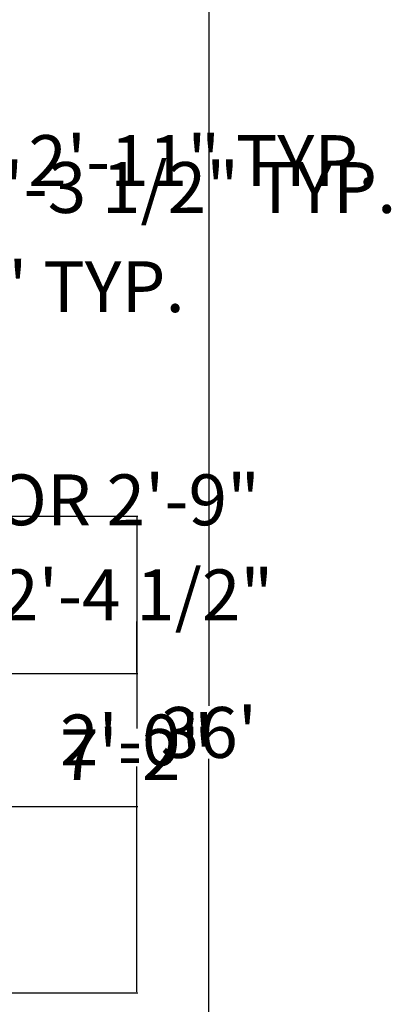
# Model space of a CAD drawing. Units: inches. Extents: x 1086 to 1540, y 3343 to 3848.
# Tile 7 of 8: x 1473 to 1540, y 3547 to 3724. Entities that reach past the tile are written whole.
import ezdxf

# ---------------------------------------------------------------- set-up
doc = ezdxf.new("R2010")
doc.units = ezdxf.units.IN
doc.layers.add('A-ANNO-DIMS', color=2, linetype='Continuous', lineweight=13)
doc.styles.get("Standard").update_dxf_attribs({"font": 'arial.ttf'})
doc.dimstyles.get("Standard").update_dxf_attribs({"dimtxt": 9.18, "dimasz": 0.18, "dimexe": 0.18, "dimexo": 0.0625, "dimgap": 0.09, "dimtad": 0, "dimtih": 1, "dimtoh": 1, "dimdec": 1, "dimzin": 0, "dimdsep": 46, "dimlunit": 3, "dimtxsty": 'Standard', "dimcen": 0.09, "dimadec": 0, "dimazin": 0, "dimtfac": 1, "dimtdec": 1, "dimtofl": 0, "dimtmove": 0, "dimatfit": 3, "dimfxl": 1, "dimtolj": 1, "dimtzin": 0, "dimarcsym": 0})

# ---------------------------------------------------------------- blocks, each defined once
blk = doc.blocks.new('*D13')
at = {"layer": 'A-ANNO-DIMS', "color": 0, "lineweight": -2, "transparency": 16777216}
for p, q in [((1470.8, 3811.57), (1506.93, 3811.57)), ((1506.75, 3811.39), (1506.75, 3600.35)), ((1506.75, 3379.75), (1506.75, 3590.79)), ((1470.8, 3379.57), (1506.93, 3379.57))]:
    blk.add_line(p, q, dxfattribs=at)
at = {"layer": 'A-ANNO-DIMS', "color": 0, "transparency": 16777216}
for points in [[(1506.72, 3811.39), (1506.78, 3811.39), (1506.75, 3811.57)], [(1506.72, 3379.75), (1506.78, 3379.75), (1506.75, 3379.57)]]:
    blk.add_solid(points, dxfattribs=at)
at = {"layer": 'Defpoints', "color": 0, "transparency": 16777216}
for p in [(1470.74, 3811.57), (1470.74, 3379.57), (1506.75, 3379.57)]:
    blk.add_point(p, dxfattribs=at)
at = {"layer": 'A-ANNO-DIMS', "color": 0, "transparency": 16777216, "insert": (1506.75, 3595.57), "char_height": 9.18, "attachment_point": 5}
blk.add_mtext("\\A1;36'", dxfattribs=at)
blk = doc.blocks.new('*D27')
at = {"layer": 'A-ANNO-DIMS', "color": 0, "lineweight": -2, "transparency": 16777216}
for p, q in [((1408.96, 3695.2), (1404.91, 3698.73)), ((1405.05, 3698.61), (1405.16, 3698.75)), ((1405.16, 3698.75), (1405.34, 3698.75)), ((1382.16, 3672.32), (1404.93, 3698.48)), ((1385.96, 3668.77), (1381.9, 3672.3))]:
    blk.add_line(p, q, dxfattribs=at)
at = {"layer": 'A-ANNO-DIMS', "color": 0, "transparency": 16777216}
for points in [[(1404.9, 3698.5), (1404.95, 3698.46), (1405.05, 3698.61)], [(1382.14, 3672.34), (1382.18, 3672.3), (1382.04, 3672.18)]]:
    blk.add_solid(points, dxfattribs=at)
at = {"layer": 'Defpoints', "color": 0, "transparency": 16777216}
for p in [(1405.05, 3698.61), (1409.01, 3695.16), (1386, 3668.73)]:
    blk.add_point(p, dxfattribs=at)
at = {"layer": 'A-ANNO-DIMS', "color": 0, "transparency": 16777216, "insert": (1473.23, 3698.75), "char_height": 9.18, "attachment_point": 5}
blk.add_mtext('\\A1;ARMCHAIR 2\'-11" TYP.', dxfattribs=at)
blk = doc.blocks.new('*D28')
at = {"layer": 'A-ANNO-DIMS', "color": 0, "lineweight": -2, "transparency": 16777216}
for p, q in [((1409.05, 3695.21), (1412.58, 3699.26)), ((1412.6, 3699.01), (1438.75, 3676.24)), ((1435.48, 3672.2), (1439.01, 3676.26)), ((1438.89, 3676.12), (1439.02, 3676)), ((1439.02, 3676), (1439.2, 3676))]:
    blk.add_line(p, q, dxfattribs=at)
at = {"layer": 'A-ANNO-DIMS', "color": 0, "transparency": 16777216}
for points in [[(1412.62, 3699.03), (1412.58, 3698.98), (1412.46, 3699.13)], [(1438.77, 3676.26), (1438.73, 3676.22), (1438.89, 3676.12)]]:
    blk.add_solid(points, dxfattribs=at)
at = {"layer": 'Defpoints', "color": 0, "transparency": 16777216}
for p in [(1409.01, 3695.16), (1438.89, 3676.12), (1435.44, 3672.16)]:
    blk.add_point(p, dxfattribs=at)
at = {"layer": 'A-ANNO-DIMS', "color": 0, "transparency": 16777216, "insert": (1470.92, 3676), "char_height": 9.18, "attachment_point": 5}
blk.add_mtext('\\A1;2\'-11" TYP.', dxfattribs=at)
blk = doc.blocks.new('*D31')
at = {"layer": 'A-ANNO-DIMS', "color": 0, "lineweight": -2, "transparency": 16777216}
for p, q in [((1461.8, 3713.61), (1467.84, 3713.61)), ((1467.66, 3713.43), (1467.66, 3698.73)), ((1467.66, 3674.34), (1467.66, 3689.04)), ((1461.8, 3674.16), (1467.84, 3674.16))]:
    blk.add_line(p, q, dxfattribs=at)
at = {"layer": 'A-ANNO-DIMS', "color": 0, "transparency": 16777216}
for points in [[(1467.63, 3713.43), (1467.69, 3713.43), (1467.66, 3713.61)], [(1467.63, 3674.34), (1467.69, 3674.34), (1467.66, 3674.16)]]:
    blk.add_solid(points, dxfattribs=at)
at = {"layer": 'Defpoints', "color": 0, "transparency": 16777216}
for p in [(1461.74, 3713.61), (1461.74, 3674.16), (1467.66, 3674.16)]:
    blk.add_point(p, dxfattribs=at)
at = {"layer": 'A-ANNO-DIMS', "color": 0, "transparency": 16777216, "insert": (1467.66, 3693.89), "char_height": 9.18, "attachment_point": 5}
blk.add_mtext('\\A1;BOOKCASE 3\'-3 1/2" TYP.', dxfattribs=at)
blk = doc.blocks.new('*D41')
at = {"layer": 'A-ANNO-DIMS', "color": 0, "lineweight": -2, "transparency": 16777216}
for p, q in [((1369.71, 3632.63), (1369.71, 3637.72)), ((1369.89, 3637.54), (1402.67, 3637.54)), ((1402.85, 3632.63), (1402.85, 3637.72)), ((1402.85, 3637.54), (1403.03, 3637.54))]:
    blk.add_line(p, q, dxfattribs=at)
at = {"layer": 'A-ANNO-DIMS', "color": 0, "transparency": 16777216}
for points in [[(1369.89, 3637.57), (1369.89, 3637.51), (1369.71, 3637.54)], [(1402.67, 3637.57), (1402.67, 3637.51), (1402.85, 3637.54)]]:
    blk.add_solid(points, dxfattribs=at)
at = {"layer": 'Defpoints', "color": 0, "transparency": 16777216}
for p in [(1402.85, 3637.54), (1369.71, 3632.57), (1402.85, 3632.57)]:
    blk.add_point(p, dxfattribs=at)
at = {"layer": 'A-ANNO-DIMS', "color": 0, "transparency": 16777216, "insert": (1460.68, 3637.54), "char_height": 9.18, "attachment_point": 5}
blk.add_mtext('\\A1;TOILET DOOR 2\'-9"', dxfattribs=at)
blk = doc.blocks.new('*D67')
at = {"layer": 'A-ANNO-DIMS', "color": 0, "lineweight": -2, "transparency": 16777216}
for p, q in [((1425.8, 3606.21), (1493.92, 3606.21)), ((1493.74, 3606.03), (1493.74, 3598.99)), ((1493.74, 3582.39), (1493.74, 3589.44)), ((1425.8, 3582.21), (1493.92, 3582.21))]:
    blk.add_line(p, q, dxfattribs=at)
at = {"layer": 'A-ANNO-DIMS', "color": 0, "transparency": 16777216}
for points in [[(1493.71, 3606.03), (1493.77, 3606.03), (1493.74, 3606.21)], [(1493.71, 3582.39), (1493.77, 3582.39), (1493.74, 3582.21)]]:
    blk.add_solid(points, dxfattribs=at)
at = {"layer": 'Defpoints', "color": 0, "transparency": 16777216}
for p in [(1425.74, 3606.21), (1493.74, 3606.21), (1425.74, 3582.21)]:
    blk.add_point(p, dxfattribs=at)
at = {"layer": 'A-ANNO-DIMS', "color": 0, "transparency": 16777216, "insert": (1493.74, 3594.21), "char_height": 9.18, "attachment_point": 5}
blk.add_mtext('\\A1;2\'-0"', dxfattribs=at)
blk = doc.blocks.new('*D68')
at = {"layer": 'A-ANNO-DIMS', "color": 0, "lineweight": -2, "transparency": 16777216}
for p, q in [((1425.8, 3634.57), (1493.92, 3634.57)), ((1493.74, 3634.39), (1493.74, 3625.23)), ((1493.74, 3606.39), (1493.74, 3615.56)), ((1425.8, 3606.21), (1493.92, 3606.21))]:
    blk.add_line(p, q, dxfattribs=at)
at = {"layer": 'A-ANNO-DIMS', "color": 0, "transparency": 16777216}
for points in [[(1493.71, 3634.39), (1493.77, 3634.39), (1493.74, 3634.57)], [(1493.71, 3606.39), (1493.77, 3606.39), (1493.74, 3606.21)]]:
    blk.add_solid(points, dxfattribs=at)
at = {"layer": 'Defpoints', "color": 0, "transparency": 16777216}
for p in [(1425.74, 3634.57), (1493.74, 3634.57), (1425.74, 3606.21)]:
    blk.add_point(p, dxfattribs=at)
at = {"layer": 'A-ANNO-DIMS', "color": 0, "transparency": 16777216, "insert": (1493.74, 3620.39), "char_height": 9.18, "attachment_point": 5}
blk.add_mtext('\\A1;2\'-4 1/2"', dxfattribs=at)
blk = doc.blocks.new('*D71')
at = {"layer": 'A-ANNO-DIMS', "color": 0, "lineweight": -2, "transparency": 16777216}
for p, q in [((1461.8, 3634.57), (1493.92, 3634.57)), ((1493.74, 3634.39), (1493.74, 3596.27)), ((1493.74, 3548.75), (1493.74, 3586.87)), ((1461.8, 3548.57), (1493.92, 3548.57))]:
    blk.add_line(p, q, dxfattribs=at)
at = {"layer": 'A-ANNO-DIMS', "color": 0, "transparency": 16777216}
for points in [[(1493.71, 3634.39), (1493.77, 3634.39), (1493.74, 3634.57)], [(1493.71, 3548.75), (1493.77, 3548.75), (1493.74, 3548.57)]]:
    blk.add_solid(points, dxfattribs=at)
at = {"layer": 'Defpoints', "color": 0, "transparency": 16777216}
for p in [(1461.74, 3634.57), (1493.74, 3634.57), (1461.74, 3548.57)]:
    blk.add_point(p, dxfattribs=at)
at = {"layer": 'A-ANNO-DIMS', "color": 0, "transparency": 16777216, "insert": (1493.74, 3591.57), "char_height": 9.18, "attachment_point": 5}
blk.add_mtext('\\A1;7\'-2"', dxfattribs=at)

msp = doc.modelspace()

# ---------------------------------------------------------------- dimensions: what is measured, and where the dimension line sits
at = {"layer": 'A-ANNO-DIMS'}
for base, p1, p2, override, picture, middle in [((1506.75, 3379.57), (1470.74, 3811.57), (1470.74, 3379.57), {"dimclrd": 0, "dimclre": 0, "dimclrt": 0}, '*D13', (1506.75, 3595.57)), ((1493.74, 3634.57), (1425.74, 3606.21), (1425.74, 3634.57), {"dimdec": 1, "dimlfac": 1, "dimrnd": 0, "dimzin": 1, "dimdsep": 46, "dimlunit": 4, "dimfrac": 2}, '*D68', (1493.74, 3620.39)), ((1493.74, 3634.57), (1461.74, 3548.57), (1461.74, 3634.57), {"dimdec": 1, "dimlfac": 1, "dimrnd": 0, "dimzin": 1, "dimdsep": 46, "dimlunit": 4, "dimfrac": 2}, '*D71', (1493.74, 3591.57)), ((1493.74, 3606.21), (1425.74, 3582.21), (1425.74, 3606.21), {"dimdec": 1, "dimlfac": 1, "dimrnd": 0, "dimzin": 1, "dimdsep": 46, "dimlunit": 4, "dimfrac": 2}, '*D67', (1493.74, 3594.21))]:
    dim = msp.add_linear_dim(base=base, p1=p1, p2=p2, angle=90, dimstyle='Standard', override=override, dxfattribs=at)
    dim.commit()
    dim.dimension.update_dxf_attribs({"geometry": picture, "text_midpoint": middle})
for base, p1, p2, angle, text, picture, middle in [((1467.6583, 3674.1617), (1461.7404, 3713.6137), (1461.7404, 3674.1617), 270, 'BOOKCASE <> TYP.', '*D31', (1467.6583, 3693.8877)), ((1405.05, 3698.61), (1386, 3668.73), (1409.01, 3695.16), 48.9613, 'ARMCHAIR <> TYP.', '*D27', (1473.23, 3698.75)), ((1438.89, 3676.12), (1409.01, 3695.16), (1435.44, 3672.16), 318.9613, '<> TYP.', '*D28', (1470.92, 3676))]:
    dim = msp.add_linear_dim(base=base, p1=p1, p2=p2, angle=angle, text=text, dimstyle='Standard', override={"dimdec": 1, "dimlfac": 1, "dimrnd": 0, "dimzin": 1, "dimdsep": 46, "dimlunit": 4, "dimfrac": 2}, dxfattribs=at)
    dim.commit()
    dim.dimension.update_dxf_attribs({"geometry": picture, "text_midpoint": middle})
dim = msp.add_linear_dim(base=(1402.85, 3637.54), p1=(1369.71, 3632.57), p2=(1402.85, 3632.57), text='TOILET DOOR <>', dimstyle='Standard', override={"dimdec": 1, "dimlfac": 1, "dimrnd": 0, "dimzin": 1, "dimdsep": 46, "dimlunit": 4, "dimfrac": 2}, dxfattribs=at)
dim.commit()
dim.dimension.update_dxf_attribs({"geometry": '*D41', "text_midpoint": (1460.68, 3637.54)})

doc.saveas('drawing.dxf')
